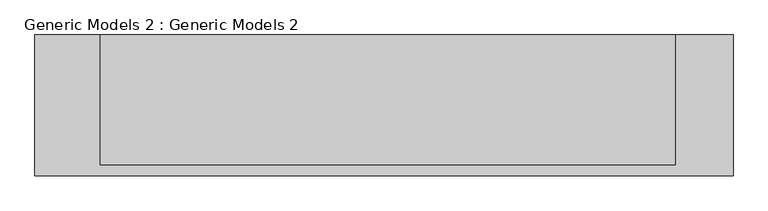
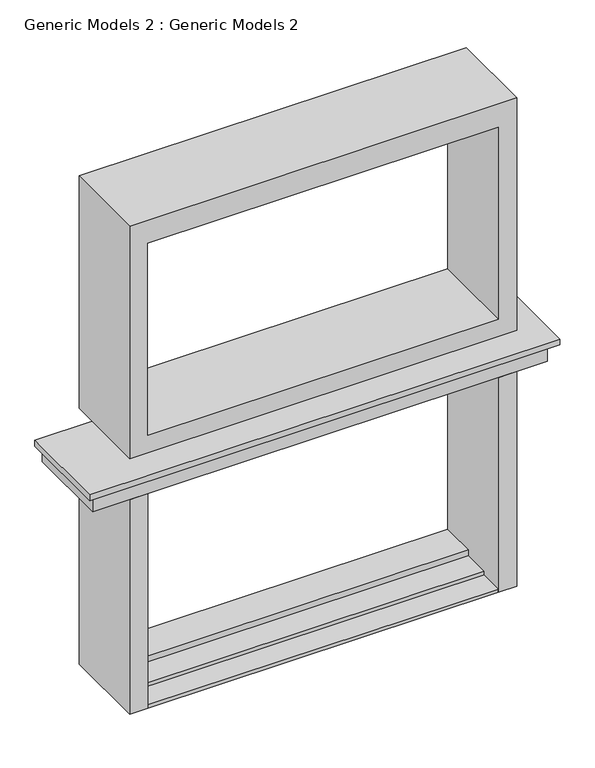
"""IFC4 building model written with IfcOpenShell, lengths in millimetres: proxy geometry, Generic Models 2 : Generic Models 2."""

from ifc_helpers import new_model, si_unit, frame, origin, origin_with_axes, place, context, project, spatial, polyline, outline, extrude, source, transform, mapped, element, save


def generic_models_2_generic_models_2_3b55f561(model_context):
    return source(origin(), model_context, "Body", "SweptSolid", [
        extrude(outline(polyline([(6400.8, -14285.1702714), (6400.8, -19085.7702714), (3352.8, -19085.7702714), (3352.8, -14285.1702714), (6400.8, -14285.1702714)]), holes=[polyline([(6096.0, -18857.1702714), (6096.0, -14513.7702714), (3581.4, -14513.7702714), (3581.4, -18857.1702714), (6096.0, -18857.1702714)])]), frame((0.0, -12672.4349955, 0.0), z_axis=(0.0, 1.0, 0.0), x_axis=(0.0, 0.0, 1.0)), (0.0, 0.0, 1.0), 1084.6966052),
        extrude(outline(polyline([(-13802.5702714, -12763.9928177), (-19633.4337496, -12763.9928177), (-19633.4337496, -11587.7383903), (-13802.5702714, -11587.7383903), (-13802.5702714, -12763.9928177)])), frame((0.0, 0.0, 3048.0), z_axis=(0.0, 0.0, 1.0), x_axis=(1.0, 0.0, 0.0)), (0.0, 0.0, 1.0), 76.2),
        extrude(outline(polyline([(-13907.6862442, -12672.4349955), (-19542.9702714, -12672.4349955), (-19542.9702714, -11587.7383903), (-13907.6862442, -11587.7383903), (-13907.6862442, -12672.4349955)])), frame((0.0, 0.0, 2814.83623), z_axis=(0.0, 0.0, 1.0), x_axis=(1.0, 0.0, 0.0)), (0.0, 0.0, 1.0), 233.16377),
        extrude(outline(polyline([(-19085.7702714, -12672.4349955), (-19085.7702714, -11587.7383903), (-18857.1702714, -11587.7383903), (-18857.1702714, -12672.4349955), (-19085.7702714, -12672.4349955)])), origin_with_axes(), (0.0, 0.0, 1.0), 2814.83623),
        extrude(outline(polyline([(-14285.1702714, -11587.7383903), (-14285.1702714, -12672.4349955), (-14513.7702714, -12672.4349955), (-14513.7702714, -11587.7383903), (-14285.1702714, -11587.7383903)])), origin_with_axes(), (0.0, 0.0, 1.0), 2814.83623),
        extrude(outline(polyline([(-14513.7702714, -12672.4349955), (-18857.1702714, -12672.4349955), (-18857.1702714, -12367.6349955), (-14513.7702714, -12367.6349955), (-14513.7702714, -12672.4349955)])), origin_with_axes(), (0.0, 0.0, 1.0), 41.3296116),
        extrude(outline(polyline([(-14513.7702714, -12367.6349955), (-18857.1702714, -12367.6349955), (-18857.1702714, -12030.6968178), (-14513.7702714, -12030.6968178), (-14513.7702714, -12367.6349955)])), origin_with_axes(), (0.0, 0.0, 1.0), 90.7760919),
        extrude(outline(polyline([(-14513.7702714, -12030.6968178), (-18857.1702714, -12030.6968178), (-18857.1702714, -11587.7383903), (-14513.7702714, -11587.7383903), (-14513.7702714, -12030.6968178)])), origin_with_axes(), (0.0, 0.0, 1.0), 167.6578856),
    ])


if __name__ == "__main__":
    model = new_model("IFC4")
    model_context = context("Model", 3, world=origin())
    ifc_project = project(units=[si_unit("LENGTHUNIT", "METRE", prefix="MILLI")], contexts=[model_context])
    site = spatial("IfcSite", under=ifc_project)
    building = spatial("IfcBuilding", under=site)
    placement = place(None, origin())
    generic_models_2_generic_models_2_shape = generic_models_2_generic_models_2_3b55f561(model_context)
    element("IfcBuildingElementProxy", 1, Name="Generic Models 2 : Generic Models 2", ObjectType="Generic Models 2 : Generic Models 2", at=placement, inside=building, context=model_context, shape_type="MappedRepresentation", body=[
        mapped(generic_models_2_generic_models_2_shape, transform((0.0, 0.0, 0.0), x_axis=(1.0, 0.0, 0.0), y_axis=(0.0, 1.0, 0.0), z_axis=(0.0, 0.0, 1.0))),
    ])
    save(model, "model.ifc")
